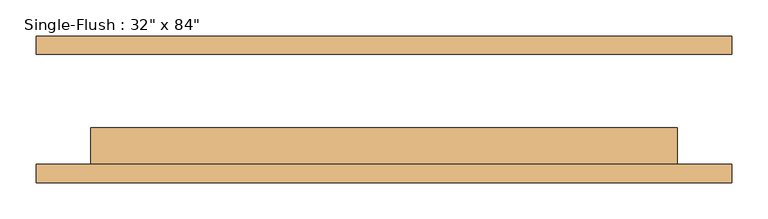
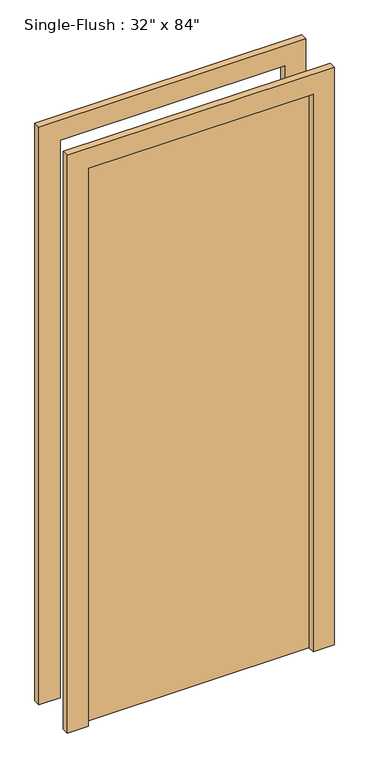
"""IFC4 building model written with IfcOpenShell, lengths in millimetres: door geometry."""

from ifc_helpers import new_model, si_unit, frame, origin, origin_with_axes, place, context, project, spatial, polyline, outline, extrude, source, transform, mapped, element, save


def door_bb092f7c(model_context):
    return source(origin(), model_context, "Body", "SweptSolid", [
        extrude(outline(polyline([(2209.8, -482.6), (0.0, -482.6), (0.0, -406.4), (2133.6, -406.4), (2133.6, 406.4), (0.0, 406.4), (0.0, 482.6), (2209.8, 482.6), (2209.8, -482.6)])), frame((0.0, -101.6, 0.0), z_axis=(0.0, 1.0, 0.0), x_axis=(0.0, 0.0, 1.0)), (0.0, 0.0, 1.0), 25.4),
        extrude(outline(polyline([(2209.8, 482.6), (2209.8, -482.6), (0.0, -482.6), (0.0, -406.4), (2133.6, -406.4), (2133.6, 406.4), (0.0, 406.4), (0.0, 482.6), (2209.8, 482.6)])), frame((0.0, 76.2, 0.0), z_axis=(0.0, 1.0, 0.0), x_axis=(0.0, 0.0, 1.0)), (0.0, 0.0, 1.0), 25.4),
        extrude(outline(polyline([(406.4, -25.4), (406.4, -76.2), (-406.4, -76.2), (-406.4, -25.4), (406.4, -25.4)])), origin_with_axes(), (0.0, 0.0, 1.0), 2133.6),
    ])


if __name__ == "__main__":
    model = new_model("IFC4")
    model_context = context("Model", 3, world=origin())
    ifc_project = project(units=[si_unit("LENGTHUNIT", "METRE", prefix="MILLI")], contexts=[model_context])
    site = spatial("IfcSite", under=ifc_project)
    building = spatial("IfcBuilding", under=site)
    placement = place(None, origin())
    door_shape = door_bb092f7c(model_context)
    element("IfcDoor", 1, ObjectType="Single-Flush : 32\" x 84\"", at=placement, inside=building, context=model_context, shape_type="MappedRepresentation", body=[
        mapped(door_shape, transform((0.0, 0.0, 0.0), x_axis=(1.0, 0.0, 0.0), y_axis=(0.0, 1.0, 0.0), z_axis=(0.0, 0.0, 1.0))),
    ])
    save(model, "model.ifc")

# Revit data of these elements
# Type "Single-Flush : 32\" x 84\""
#   Type Mark = "3"
#   Construction Type Id = "MDOOR"
#   Assembly Code = "C1020"
#   Analytic Construction = "Metal"
#   Thickness = 0' - 2"
#   Heat Transfer Coefficient (U) = 0.651978 BTU/(h·ft²·°F)
#   Height = 7' - 0"
#   Trim Projection Ext = 0' - 1"
#   Trim Projection Int = 0' - 1"
#   Trim Width = 0' - 3"
#   Width = 2' - 8"
#   Define Thermal Properties by = 1
#   Door Material = Door - Panel
#   Frame Material = Door - Frame
#   Visual Light Transmittance = 0
#   Solar Heat Gain Coefficient = 0
#   Function = (empty or 0)
#   Wall Closure = (empty or 0)
# Element 1 (IfcDoor, "Single-Flush : 32\" x 84\"")
#   Materials on its faces: "Door - Frame", "Door - Panel"
# Materials
#   "Door - Panel": class "Wood", colour RGB 210 159 95, transparency 0
#   "Door - Frame": colour RGB 118 70 51, transparency 0
